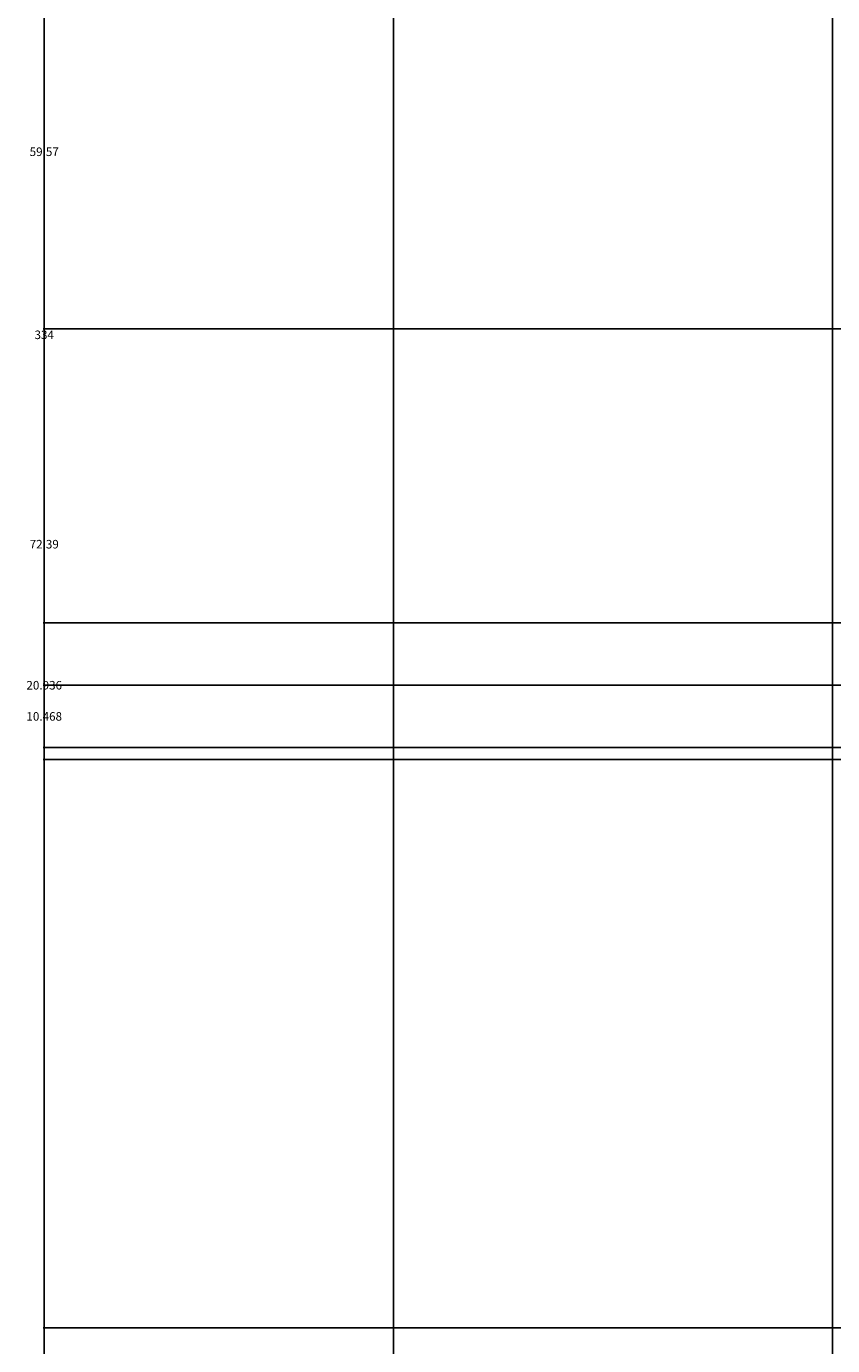
# Model space of a CAD drawing. Units: inches. Extents: x 241 to 943, y 109 to 1396.
# Tile 6 of 34: x 241 to 377, y 398 to 620. Entities that reach past the tile are written whole.
import ezdxf

# ---------------------------------------------------------------- set-up
doc = ezdxf.new("R2010")
doc.units = ezdxf.units.IN
doc.header["$MEASUREMENT"] = 0
doc.layers.add('A-ANNO-DIMS', color=2, linetype='Continuous', lineweight=18)
doc.styles.get("Standard").update_dxf_attribs({"font": 'arial.ttf'})
doc.dimstyles.get("Standard").update_dxf_attribs({"dimtxt": 1.4375, "dimasz": 0.18, "dimexe": 0.18, "dimexo": 0.0625, "dimgap": 0.09, "dimtad": 0, "dimtih": 1, "dimtoh": 1, "dimdec": 4, "dimzin": 0, "dimdsep": 46, "dimlunit": 4, "dimtxsty": 'Standard', "dimcen": 0.09, "dimadec": 0, "dimazin": 0, "dimtfac": 1, "dimtdec": 4, "dimtofl": 0, "dimtmove": 0, "dimatfit": 3, "dimfxl": 1, "dimtolj": 1, "dimtzin": 0, "dimarcsym": 0})

# ---------------------------------------------------------------- blocks, each defined once
blk = doc.blocks.new('*D5')
at = {"layer": 'A-ANNO-DIMS', "color": 0, "lineweight": -2, "transparency": 16777216}
for p, q in [((303.24, 177.8), (303.24, 1395.05)), ((303.42, 1394.87), (338.18, 1394.87)), ((376.86, 1394.87), (342.09, 1394.87)), ((377.04, 177.76), (377.04, 1395.05))]:
    blk.add_line(p, q, dxfattribs=at)
at = {"layer": 'A-ANNO-DIMS', "color": 0, "transparency": 16777216}
for points in [[(303.42, 1394.9), (303.42, 1394.84), (303.24, 1394.87)], [(376.86, 1394.9), (376.86, 1394.84), (377.04, 1394.87)]]:
    blk.add_solid(points, dxfattribs=at)
at = {"layer": 'Defpoints', "color": 0, "transparency": 16777216}
for p in [(377.04, 1394.87), (303.24, 177.74), (377.04, 177.7)]:
    blk.add_point(p, dxfattribs=at)
at = {"layer": 'A-ANNO-DIMS', "color": 0, "transparency": 16777216, "insert": (340.14, 1394.87), "char_height": 1.438, "attachment_point": 5}
blk.add_mtext('\\A1;73.8', dxfattribs=at)
blk = doc.blocks.new('*D7')
at = {"layer": 'A-ANNO-DIMS', "color": 0, "lineweight": -2, "transparency": 16777216}
for p, q in [((508.24, 1336.12), (244.31, 1336.12)), ((244.49, 1335.94), (244.49, 753.25)), ((244.49, 168.92), (244.49, 751.6)), ((303.17, 168.74), (244.31, 168.74))]:
    blk.add_line(p, q, dxfattribs=at)
at = {"layer": 'A-ANNO-DIMS', "color": 0, "transparency": 16777216}
for points in [[(244.46, 1335.94), (244.52, 1335.94), (244.49, 1336.12)], [(244.46, 168.92), (244.52, 168.92), (244.49, 168.74)]]:
    blk.add_solid(points, dxfattribs=at)
at = {"layer": 'Defpoints', "color": 0, "transparency": 16777216}
for p in [(244.49, 1336.12), (508.31, 1336.12), (303.24, 168.74)]:
    blk.add_point(p, dxfattribs=at)
at = {"layer": 'A-ANNO-DIMS', "color": 0, "transparency": 16777216, "insert": (244.49, 752.43), "char_height": 1.438, "attachment_point": 5}
blk.add_mtext('\\A1;1167.4', dxfattribs=at)
blk = doc.blocks.new('*D8')
at = {"layer": 'A-ANNO-DIMS', "color": 0, "lineweight": -2, "transparency": 16777216}
for p, q in [((377.04, 396.94), (377.04, 1395.05)), ((377.22, 1394.87), (380.96, 1394.87)), ((390.71, 1394.87), (386.97, 1394.87)), ((390.89, 384.24), (390.89, 1395.05))]:
    blk.add_line(p, q, dxfattribs=at)
at = {"layer": 'A-ANNO-DIMS', "color": 0, "transparency": 16777216}
for points in [[(377.22, 1394.9), (377.22, 1394.84), (377.04, 1394.87)], [(390.71, 1394.9), (390.71, 1394.84), (390.89, 1394.87)]]:
    blk.add_solid(points, dxfattribs=at)
at = {"layer": 'Defpoints', "color": 0, "transparency": 16777216}
for p in [(390.89, 1394.87), (377.04, 396.88), (390.89, 384.18)]:
    blk.add_point(p, dxfattribs=at)
at = {"layer": 'A-ANNO-DIMS', "color": 0, "transparency": 16777216, "insert": (383.97, 1394.87), "char_height": 1.438, "attachment_point": 5}
blk.add_mtext('\\A1;13.856', dxfattribs=at)
blk = doc.blocks.new('*D20')
at = {"layer": 'A-ANNO-DIMS', "color": 0, "lineweight": -2, "transparency": 16777216}
for p, q in [((376.98, 400.83), (244.31, 400.83)), ((244.49, 400.65), (244.49, 290.09)), ((244.49, 177.88), (244.49, 288.44)), ((376.98, 177.7), (244.31, 177.7))]:
    blk.add_line(p, q, dxfattribs=at)
at = {"layer": 'A-ANNO-DIMS', "color": 0, "transparency": 16777216}
for points in [[(244.46, 400.65), (244.52, 400.65), (244.49, 400.83)], [(244.46, 177.88), (244.52, 177.88), (244.49, 177.7)]]:
    blk.add_solid(points, dxfattribs=at)
at = {"layer": 'Defpoints', "color": 0, "transparency": 16777216}
for p in [(244.49, 400.83), (377.04, 400.83), (377.04, 177.7)]:
    blk.add_point(p, dxfattribs=at)
at = {"layer": 'A-ANNO-DIMS', "color": 0, "transparency": 16777216, "insert": (244.49, 289.26), "char_height": 1.438, "attachment_point": 5}
blk.add_mtext('\\A1;223.13', dxfattribs=at)
blk = doc.blocks.new('*D21')
at = {"layer": 'A-ANNO-DIMS', "color": 0, "lineweight": -2, "transparency": 16777216}
for p, q in [((376.98, 734.85), (244.31, 734.85)), ((244.49, 734.67), (244.49, 568.67)), ((244.49, 401.01), (244.49, 567.02)), ((376.98, 400.83), (244.31, 400.83))]:
    blk.add_line(p, q, dxfattribs=at)
at = {"layer": 'A-ANNO-DIMS', "color": 0, "transparency": 16777216}
for points in [[(244.46, 734.67), (244.52, 734.67), (244.49, 734.85)], [(244.46, 401.01), (244.52, 401.01), (244.49, 400.83)]]:
    blk.add_solid(points, dxfattribs=at)
at = {"layer": 'Defpoints', "color": 0, "transparency": 16777216}
for p in [(244.49, 734.85), (377.04, 734.85), (377.04, 400.83)]:
    blk.add_point(p, dxfattribs=at)
at = {"layer": 'A-ANNO-DIMS', "color": 0, "transparency": 16777216, "insert": (244.49, 567.84), "char_height": 1.438, "attachment_point": 5}
blk.add_mtext('\\A1;334', dxfattribs=at)
blk = doc.blocks.new('*D32')
at = {"layer": 'A-ANNO-DIMS', "color": 0, "lineweight": -2, "transparency": 16777216}
for p, q in [((424.05, 568.83), (244.31, 568.83)), ((244.49, 568.65), (244.49, 533.46)), ((244.49, 496.62), (244.49, 531.81)), ((424.05, 496.44), (244.31, 496.44))]:
    blk.add_line(p, q, dxfattribs=at)
at = {"layer": 'A-ANNO-DIMS', "color": 0, "transparency": 16777216}
for points in [[(244.46, 568.65), (244.52, 568.65), (244.49, 568.83)], [(244.46, 496.62), (244.52, 496.62), (244.49, 496.44)]]:
    blk.add_solid(points, dxfattribs=at)
at = {"layer": 'Defpoints', "color": 0, "transparency": 16777216}
for p in [(244.49, 568.83), (424.11, 568.83), (424.11, 496.44)]:
    blk.add_point(p, dxfattribs=at)
at = {"layer": 'A-ANNO-DIMS', "color": 0, "transparency": 16777216, "insert": (244.49, 532.63), "char_height": 1.438, "attachment_point": 5}
blk.add_mtext('\\A1;72.39', dxfattribs=at)
blk = doc.blocks.new('*D33')
at = {"layer": 'A-ANNO-DIMS', "color": 0, "lineweight": -2, "transparency": 16777216}
for p, q in [((424.05, 628.4), (244.31, 628.4)), ((244.49, 628.22), (244.49, 599.44)), ((244.49, 569.01), (244.49, 597.79)), ((424.05, 568.83), (244.31, 568.83))]:
    blk.add_line(p, q, dxfattribs=at)
at = {"layer": 'A-ANNO-DIMS', "color": 0, "transparency": 16777216}
for points in [[(244.46, 628.22), (244.52, 628.22), (244.49, 628.4)], [(244.46, 569.01), (244.52, 569.01), (244.49, 568.83)]]:
    blk.add_solid(points, dxfattribs=at)
at = {"layer": 'Defpoints', "color": 0, "transparency": 16777216}
for p in [(244.49, 628.4), (424.11, 628.4), (424.11, 568.83)]:
    blk.add_point(p, dxfattribs=at)
at = {"layer": 'A-ANNO-DIMS', "color": 0, "transparency": 16777216, "insert": (244.49, 598.62), "char_height": 1.438, "attachment_point": 5}
blk.add_mtext('\\A1;59.57', dxfattribs=at)
blk = doc.blocks.new('*D41')
at = {"layer": 'A-ANNO-DIMS', "color": 0, "lineweight": -2, "transparency": 16777216}
for p, q in [((820.77, 400.83), (244.31, 400.83)), ((244.49, 400.65), (244.49, 317.65)), ((244.49, 233.01), (244.49, 316.01)), ((820.77, 232.83), (244.31, 232.83))]:
    blk.add_line(p, q, dxfattribs=at)
at = {"layer": 'A-ANNO-DIMS', "color": 0, "transparency": 16777216}
for points in [[(244.46, 400.65), (244.52, 400.65), (244.49, 400.83)], [(244.46, 233.01), (244.52, 233.01), (244.49, 232.83)]]:
    blk.add_solid(points, dxfattribs=at)
at = {"layer": 'Defpoints', "color": 0, "transparency": 16777216}
for p in [(244.49, 400.83), (820.84, 400.83), (820.84, 232.83)]:
    blk.add_point(p, dxfattribs=at)
at = {"layer": 'A-ANNO-DIMS', "color": 0, "transparency": 16777216, "insert": (244.49, 316.83), "char_height": 1.438, "attachment_point": 5}
blk.add_mtext('\\A1;168', dxfattribs=at)
blk = doc.blocks.new('*D61')
at = {"layer": 'A-ANNO-DIMS', "color": 0, "lineweight": -2, "transparency": 16777216}
for p, q in [((377.04, 400.89), (377.04, 1395.05)), ((377.22, 1394.87), (398.03, 1394.87)), ((423.93, 1394.87), (403.12, 1394.87)), ((424.11, 568.89), (424.11, 1395.05))]:
    blk.add_line(p, q, dxfattribs=at)
at = {"layer": 'A-ANNO-DIMS', "color": 0, "transparency": 16777216}
for points in [[(377.22, 1394.9), (377.22, 1394.84), (377.04, 1394.87)], [(423.93, 1394.9), (423.93, 1394.84), (424.11, 1394.87)]]:
    blk.add_solid(points, dxfattribs=at)
at = {"layer": 'Defpoints', "color": 0, "transparency": 16777216}
for p in [(424.11, 1394.87), (424.11, 568.83), (377.04, 400.83)]:
    blk.add_point(p, dxfattribs=at)
at = {"layer": 'A-ANNO-DIMS', "color": 0, "transparency": 16777216, "insert": (400.57, 1394.87), "char_height": 1.438, "attachment_point": 5}
blk.add_mtext('\\A1;47.07', dxfattribs=at)
blk = doc.blocks.new('*D91')
at = {"layer": 'A-ANNO-DIMS', "color": 0, "lineweight": -2, "transparency": 16777216}
for p, q in [((377.04, 1070.79), (377.04, 109.81)), ((389.04, 1070.79), (389.04, 109.81)), ((377.22, 109.99), (380.04, 109.99)), ((388.86, 109.99), (386.04, 109.99))]:
    blk.add_line(p, q, dxfattribs=at)
at = {"layer": 'A-ANNO-DIMS', "color": 0, "transparency": 16777216}
for points in [[(377.22, 110.02), (377.22, 109.96), (377.04, 109.99)], [(388.86, 110.02), (388.86, 109.96), (389.04, 109.99)]]:
    blk.add_solid(points, dxfattribs=at)
at = {"layer": 'Defpoints', "color": 0, "transparency": 16777216}
for p in [(377.04, 1070.85), (389.04, 1070.85), (389.04, 109.99)]:
    blk.add_point(p, dxfattribs=at)
at = {"layer": 'A-ANNO-DIMS', "color": 0, "transparency": 16777216, "insert": (383.04, 109.99), "char_height": 1.438, "attachment_point": 5}
blk.add_mtext('\\A1;12.004', dxfattribs=at)
blk = doc.blocks.new('*D140')
at = {"layer": 'A-ANNO-DIMS', "color": 0, "lineweight": -2, "transparency": 16777216}
for p, q in [((446.37, 519.38), (244.31, 519.38)), ((244.49, 519.2), (244.49, 509.73)), ((244.49, 498.62), (244.49, 508.08)), ((446.37, 498.44), (244.31, 498.44))]:
    blk.add_line(p, q, dxfattribs=at)
at = {"layer": 'A-ANNO-DIMS', "color": 0, "transparency": 16777216}
for points in [[(244.46, 519.2), (244.52, 519.2), (244.49, 519.38)], [(244.46, 498.62), (244.52, 498.62), (244.49, 498.44)]]:
    blk.add_solid(points, dxfattribs=at)
at = {"layer": 'Defpoints', "color": 0, "transparency": 16777216}
for p in [(244.49, 519.38), (446.43, 519.38), (446.43, 498.44)]:
    blk.add_point(p, dxfattribs=at)
at = {"layer": 'A-ANNO-DIMS', "color": 0, "transparency": 16777216, "insert": (244.49, 508.91), "char_height": 1.438, "attachment_point": 5}
blk.add_mtext('\\A1;20.936', dxfattribs=at)
blk = doc.blocks.new('*D141')
at = {"layer": 'A-ANNO-DIMS', "color": 0, "lineweight": -2, "transparency": 16777216}
for p, q in [((508.13, 508.91), (244.31, 508.91)), ((244.49, 508.73), (244.49, 504.5)), ((244.49, 498.62), (244.49, 502.85)), ((508.13, 498.44), (244.31, 498.44))]:
    blk.add_line(p, q, dxfattribs=at)
at = {"layer": 'A-ANNO-DIMS', "color": 0, "transparency": 16777216}
for points in [[(244.46, 508.73), (244.52, 508.73), (244.49, 508.91)], [(244.46, 498.62), (244.52, 498.62), (244.49, 498.44)]]:
    blk.add_solid(points, dxfattribs=at)
at = {"layer": 'Defpoints', "color": 0, "transparency": 16777216}
for p in [(244.49, 508.91), (508.19, 508.91), (508.19, 498.44)]:
    blk.add_point(p, dxfattribs=at)
at = {"layer": 'A-ANNO-DIMS', "color": 0, "transparency": 16777216, "insert": (244.49, 503.67), "char_height": 1.438, "attachment_point": 5}
blk.add_mtext('\\A1;10.468', dxfattribs=at)

msp = doc.modelspace()

# ---------------------------------------------------------------- dimensions: what is measured, and where the dimension line sits
at = {"layer": 'A-ANNO-DIMS'}
for base, p1, p2, override, picture, middle in [((377.0391, 1394.8654), (303.2358, 177.7407), (377.0391, 177.6977), {"dimdec": 1, "dimlfac": 1, "dimrnd": 0, "dimzin": 0, "dimdsep": 46, "dimlunit": 2}, '*D5', (340.1375, 1394.8654)), ((390.895, 1394.8654), (377.0391, 396.8782), (390.895, 384.1784), {"dimdec": 3, "dimlfac": 1, "dimrnd": 0, "dimzin": 0, "dimdsep": 46, "dimlunit": 2}, '*D8', (383.9671, 1394.8654)), ((424.1086, 1394.8654), (377.0391, 400.8295), (424.1086, 568.8295), {"dimdec": 2, "dimlfac": 1, "dimrnd": 0, "dimzin": 0, "dimdsep": 46, "dimlunit": 2}, '*D61', (400.5739, 1394.8654)), ((389.0429, 109.9907), (377.0391, 1070.8538), (389.0429, 1070.8538), {"dimdec": 3, "dimlfac": 1, "dimrnd": 0, "dimzin": 0, "dimdsep": 46, "dimlunit": 2}, '*D91', (383.041, 109.9907))]:
    dim = msp.add_linear_dim(base=base, p1=p1, p2=p2, dimstyle='Standard', override=override, dxfattribs=at)
    dim.commit()
    dim.dimension.update_dxf_attribs({"geometry": picture, "text_midpoint": middle})
for base, p1, p2, override, picture, middle in [((244.4858, 1336.1154), (303.2358, 168.7407), (508.3064, 1336.1154), {"dimdec": 1, "dimlfac": 1, "dimrnd": 0, "dimzin": 0, "dimdsep": 46, "dimlunit": 2}, '*D7', (244.4858, 752.4281)), ((244.4858, 734.8538), (377.0391, 400.8295), (377.0391, 734.8538), {"dimdec": 0, "dimlfac": 1, "dimrnd": 0, "dimzin": 0, "dimdsep": 46, "dimlunit": 2}, '*D21', (244.4858, 567.8417)), ((244.4858, 628.4013), (424.1086, 568.8295), (424.1086, 628.4013), {"dimdec": 2, "dimlfac": 1, "dimrnd": 0, "dimzin": 0, "dimdsep": 46, "dimlunit": 2}, '*D33', (244.4858, 598.6154)), ((244.4858, 568.8295), (424.1086, 496.4395), (424.1086, 568.8295), {"dimdec": 2, "dimlfac": 1, "dimrnd": 0, "dimzin": 0, "dimdsep": 46, "dimlunit": 2}, '*D32', (244.4858, 532.6345)), ((244.4858, 519.3754), (446.4348, 498.4395), (446.4348, 519.3754), {"dimdec": 3, "dimlfac": 1, "dimrnd": 0, "dimzin": 0, "dimdsep": 46, "dimlunit": 2}, '*D140', (244.4858, 508.9074)), ((244.4858, 508.9074), (508.1906, 498.4395), (508.1906, 508.9074), {"dimdec": 3, "dimlfac": 1, "dimrnd": 0, "dimzin": 0, "dimdsep": 46, "dimlunit": 2}, '*D141', (244.4858, 503.6735)), ((244.4858, 400.8295), (377.0391, 177.6977), (377.0391, 400.8295), {"dimdec": 2, "dimlfac": 1, "dimrnd": 0, "dimzin": 0, "dimdsep": 46, "dimlunit": 2}, '*D20', (244.4858, 289.2636)), ((244.4858, 400.8295), (820.8374, 232.8295), (820.8374, 400.8295), {"dimdec": 0, "dimlfac": 1, "dimrnd": 0, "dimzin": 0, "dimdsep": 46, "dimlunit": 2}, '*D41', (244.4858, 316.8295))]:
    dim = msp.add_linear_dim(base=base, p1=p1, p2=p2, angle=90, dimstyle='Standard', override=override, dxfattribs=at)
    dim.commit()
    dim.dimension.update_dxf_attribs({"geometry": picture, "text_midpoint": middle})

doc.saveas('drawing.dxf')
